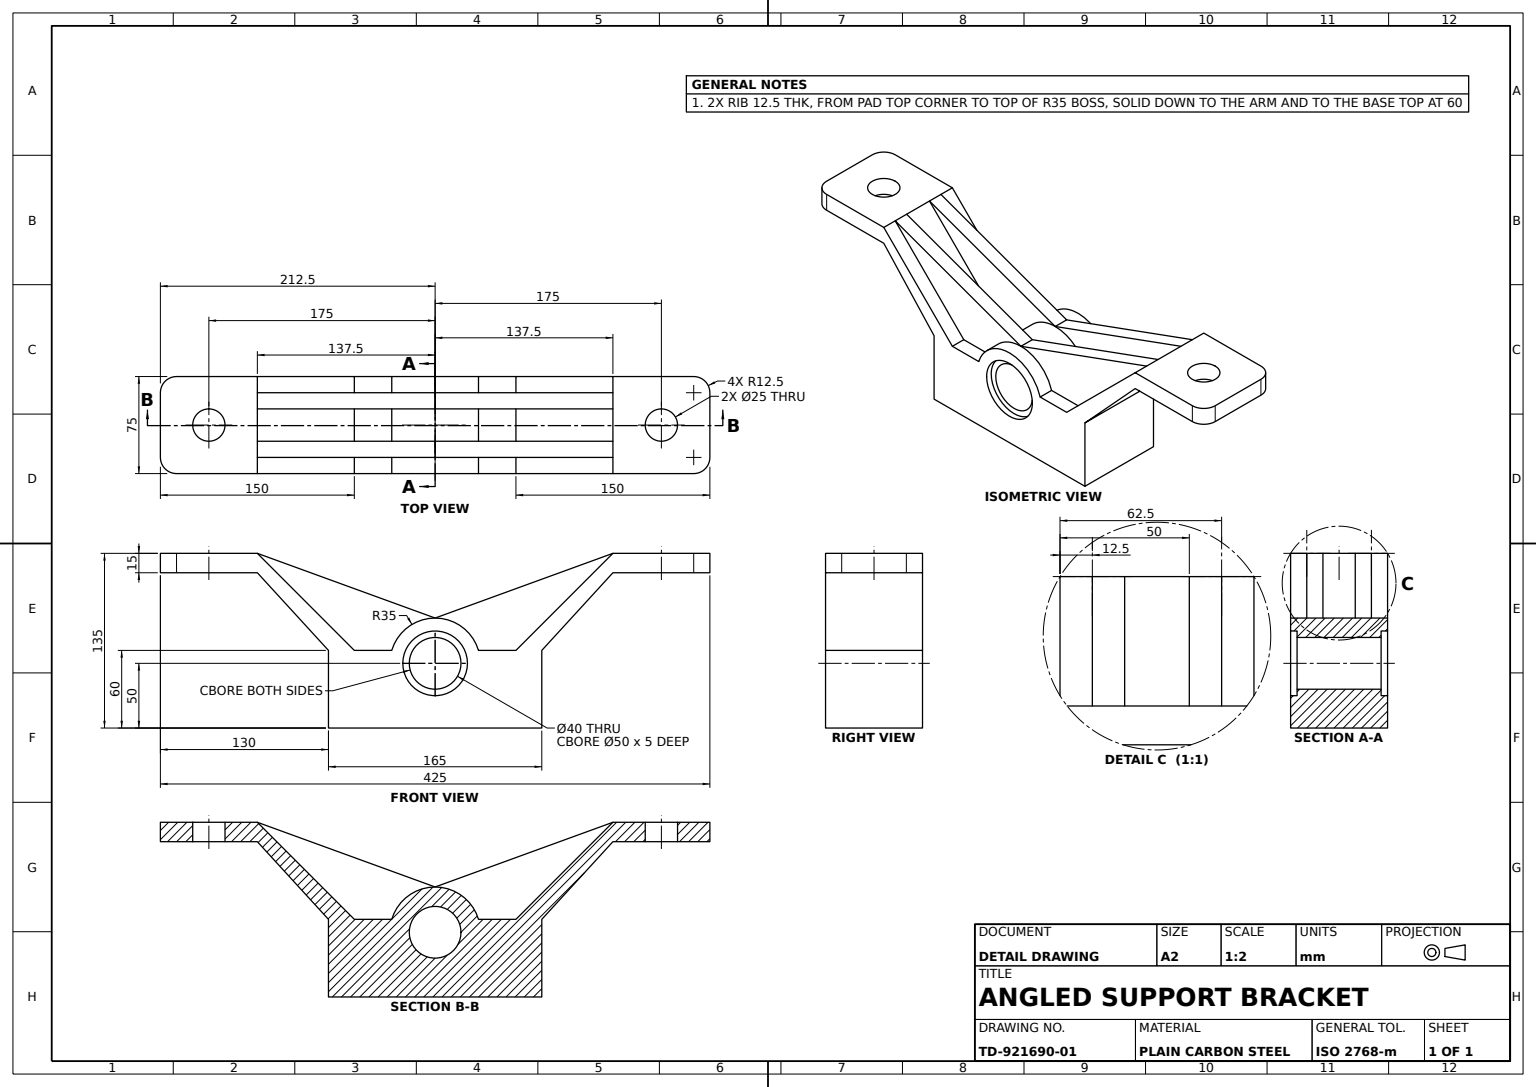
SolidWorks part; units mm, degrees
material "Plain Carbon Steel"
ref_plane "Front Plane" through (0, 0, 0) normal (0, 0, 1) x (1, 0, 0)
ref_plane "Top Plane" through (0, 0, 0) normal (0, 1, 0) x (1, 0, 0)
ref_plane "Right Plane" through (0, 0, 0) normal (1, 0, 0) x (0, 0, -1)
sketch "Support Profile Sketch" plane through (0, 0, 0) normal (0, 0, 1) x (1, 0, 0)
  line L0 (33.541, 30) -> (62.5, 30)
  line L1 (82.5, 0) -> (82.5, 30)
  line L2 (62.5, 30) -> (33.541, 30)
  line L3 (-82.5, 30) -> (-82.5, -30)
  line L4 (-82.5, -30) -> (82.5, -30)
  line L5 (82.5, -30) -> (82.5, 0)
  line L6 (62.5, 30) -> (137.5, 105)
  line L8 (-82.5, 30) -> (-137.5, 90)
  line L9 (-212.5, 105) -> (-212.5, 90)
  line L10 (82.5, 30) -> (137.5, 90)
  line L11 (137.5, 105) -> (212.5, 105)
  line L12 (212.5, 105) -> (212.5, 90)
  line L13 (212.5, 90) -> (137.5, 90)
  line L14 (-212.5, 90) -> (-137.5, 90)
  line L15 (-137.5, 105) -> (-212.5, 105)
  line L16 (-62.5, 30) -> (-137.5, 105)
  line L17 (-33.541, 30) -> (-62.5, 30)
  arc A0 (33.541, 30) -> (-33.541, 30) centre (0, 20) ccw
  dimension "D1" = 35
  dimension "D2" = 20
  dimension "D3" = 62.5
  dimension "D4" = 60
  dimension "D5" = 30
  dimension "D6" = 75
  dimension "D7" = 22.981
  dimension "D8" = 15
  dimension "D9" = 75
  dimension "D10" = 55
  dimension "D11" = 40.5435
  dimension "D12" = 60
  dimension "D13" = 165
  dimension "D14" = 75
  dimension "D15" = 75
  dimension "D16" = 22.981
  dimension "D17" = 60
  dimension "D18" = 55
  dimension "D19" = 40.5435
  dimension "D20" = 75
  dimension "D21" = 15
  dimension "D22" = 75
  dimension "D23" = 212.5
extrude "Support Body" add sketch "Support Profile Sketch" against normal blind 75 contours L0 A0 L17 L16 L15 L9 L14 L8 L3 L4 L5 L1 L10 L13 L12 L11 L6
ref_plane "Plane1" through (0, 0, -12.5) normal (0, 0, 1) x (1, 0, 0)
sketch "Rib Front Sketch" plane through (0, 0, -12.5) normal (0, 0, 1) x (1, 0, 0)
  line L0 (0, 55) -> (137.5, 105)
  line L1 (137.5, 105) -> (62.5, 30)
  line L2 (62.5, 30) -> (33.541, 30)
  line L4 (-62.5, 30) -> (-33.541, 30)
  line L5 (-137.5, 105) -> (-62.5, 30)
  line L6 (0, 55) -> (-137.5, 105)
  arc A1 (33.541, 30) -> (-33.541, 30) centre (0, 20) ccw
  dimension "D1" = 146.3087
  dimension "D2" = 137.5
  dimension "D3" = 50
  dimension "D4" = 137.5
  dimension "D5" = 75
  dimension "D6" = 75
  dimension "D7" = 28.959
extrude "Rib Front" add sketch "Rib Front Sketch" against normal blind 12.5 contours A1 L2 L1 L0 | A1 L6 L5 L4
ref_plane "Plane2" through (0, 0, -62.5) normal (0, 0, -1) x (-1, 0, 0)
sketch "Rib Back Sketch" plane through (0, 0, -62.5) normal (0, 0, -1) x (-1, 0, 0)
  line L0 (-137.5, 105) -> (-62.5, 30)
  line L1 (-62.5, 30) -> (-33.541, 30)
  line L2 (33.541, 30) -> (62.5, 30)
  line L3 (62.5, 30) -> (137.5, 105)
  line L4 (137.5, 105) -> (0, 55)
  line L5 (0, 55) -> (-137.5, 105)
  arc A0 (33.541, 30) -> (-33.541, 30) centre (0, 20) ccw
extrude "Rib Back" add sketch "Rib Back Sketch" against normal blind 12.5 contours A0 L2 L3 L4 | A0 L5 L0 L1
sketch "Mounting Holes Sketch" plane through (0, 105, 0) normal (0, 1, 0) x (1, 0, 0)
  circle A0 centre (175, 37.5) radius 12.5
  circle A1 centre (-175, 37.5) radius 12.5
  dimension "D1" = 25
  dimension "D2" = 25
  dimension "D3" = 175
  dimension "D4" = 37.5
  dimension "D5" = 175
  dimension "D6" = 37.5
extrude "Mounting Holes 2xØ25" cut sketch "Mounting Holes Sketch" against normal blind 108.5
fillet "Flange Fillet R12.5 A" radius 12.5 1 edges at (212.5, 97.5, 0)
fillet "Flange Fillet R12.5 B" radius 12.5 1 edges at (212.5, 97.5, -75)
fillet "Flange Fillet R12.5 C" radius 12.5 1 edges at (-212.5, 97.5, -75)
fillet "Flange Fillet R12.5 D" radius 12.5 1 edges at (-212.5, 97.5, 0)
sketch "Counterbore Front Sketch" plane through (0, 0, 0) normal (0, 0, 1) x (1, 0, 0)
  circle A1 centre (0, 20) radius 25
  dimension "D1" = 50
extrude "Counterbore Front Ø50x5" cut sketch "Counterbore Front Sketch" against normal blind 5
sketch "Shaft Bore Sketch" plane through (0, 0, -5) normal (0, 0, 1) x (1, 0, 0)
  circle A0 centre (0, 20) radius 20
  dimension "D1" = 40
extrude "Shaft Bore Ø40" cut sketch "Shaft Bore Sketch" against normal blind 98
sketch "Counterbore Back Sketch" plane through (0, 0, -75) normal (0, 0, -1) x (-1, 0, 0)
  circle A0 centre (0, 20) radius 25
  dimension "D1" = 50
extrude "Counterbore Back Ø50x5" cut sketch "Counterbore Back Sketch" against normal blind 5
